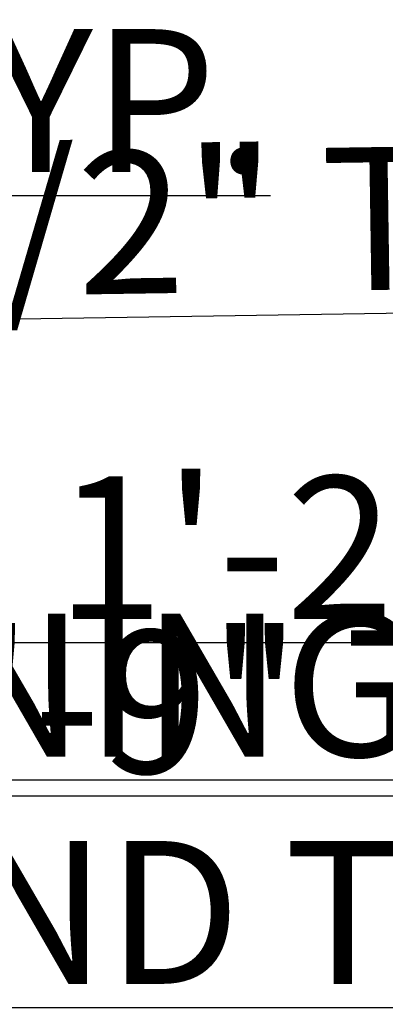
# Model space of a CAD drawing. Units: inches. Extents: x 2901 to 21549, y 2042 to 3828.
# Tile 7 of 10: x 3682 to 3774, y 3099 to 3347. Entities that reach past the tile are written whole.
import ezdxf

# ---------------------------------------------------------------- set-up
doc = ezdxf.new("R2010")
doc.units = ezdxf.units.IN
doc.layers.get('Defpoints').update_dxf_attribs({"color": 1})
doc.layers.add('A-ANNO-DIMS', color=2, linetype='Continuous', lineweight=18)
doc.styles.get("Standard").update_dxf_attribs({"font": 'arial.ttf'})
doc.dimstyles.new('ISO-25', dxfattribs={"dimtxt": 36, "dimasz": 5, "dimexe": 1.25, "dimexo": 0.625, "dimtad": 1, "dimdec": 0, "dimlunit": 3, "dimtxsty": 'Standard', "dimcen": 2.5, "dimadec": 0, "dimazin": 0, "dimtfac": 1, "dimtdec": 0, "dimtmove": 0, "dimatfit": 3, "dimfxl": 1, "dimarcsym": 0})

# ---------------------------------------------------------------- blocks, each defined once
blk = doc.blocks.new('*D36')
at = {"layer": 'A-ANNO-DIMS', "color": 0, "lineweight": -2, "transparency": 16777216}
for p, q in [((3639.47, 3192.64), (3639.47, 3654.44)), ((3634.69, 3192.64), (3640.72, 3192.64)), ((3639.47, 3161.64), (3639.47, 3187.64)), ((3634.69, 3156.64), (3640.72, 3156.64))]:
    blk.add_line(p, q, dxfattribs=at)
at = {"layer": 'A-ANNO-DIMS', "color": 0, "transparency": 16777216}
for points in [[(3638.64, 3187.64), (3640.3, 3187.64), (3639.47, 3192.64)], [(3638.64, 3161.64), (3640.3, 3161.64), (3639.47, 3156.64)]]:
    blk.add_solid(points, dxfattribs=at)
at = {"layer": 'Defpoints', "color": 0, "transparency": 16777216}
for p in [(3634.07, 3192.64), (3639.47, 3192.64), (3634.07, 3156.64)]:
    blk.add_point(p, dxfattribs=at)
at = {"layer": 'A-ANNO-DIMS', "color": 0, "transparency": 16777216, "insert": (3620.21, 3426.04), "char_height": 36, "attachment_point": 5, "rotation": 90}
blk.add_mtext('WINDOW 3\'-0" TYP.', dxfattribs=at)
blk = doc.blocks.new('*D37')
at = {"layer": 'A-ANNO-DIMS', "color": 0, "lineweight": -2, "transparency": 16777216}
for p, q in [((3625.07, 3156.01), (3625.07, 3149.99)), ((3634.07, 3156.01), (3634.07, 3149.99)), ((3620.07, 3151.24), (3615.07, 3151.24)), ((3625.07, 3151.24), (3634.07, 3151.24)), ((3639.07, 3151.24), (3864.76, 3151.24))]:
    blk.add_line(p, q, dxfattribs=at)
at = {"layer": 'A-ANNO-DIMS', "color": 0, "transparency": 16777216}
for points in [[(3620.07, 3152.07), (3620.07, 3150.41), (3625.07, 3151.24)], [(3639.07, 3152.07), (3639.07, 3150.41), (3634.07, 3151.24)]]:
    blk.add_solid(points, dxfattribs=at)
at = {"layer": 'Defpoints', "color": 0, "transparency": 16777216}
for p in [(3625.07, 3156.64), (3634.07, 3156.64), (3634.07, 3151.24)]:
    blk.add_point(p, dxfattribs=at)
at = {"layer": 'A-ANNO-DIMS', "color": 0, "transparency": 16777216, "insert": (3754.41, 3170.24), "char_height": 36, "attachment_point": 5}
blk.add_mtext('0\'-9" TYP.', dxfattribs=at)
blk = doc.blocks.new('*D38')
at = {"layer": 'A-ANNO-DIMS', "color": 0, "lineweight": -2, "transparency": 16777216}
for p, q in [((3343.07, 3191.34), (3343.07, 3188.58)), ((3357.29, 3191.34), (3357.29, 3188.58)), ((3348.07, 3189.83), (3352.29, 3189.83)), ((3357.29, 3189.83), (3922.11, 3189.83))]:
    blk.add_line(p, q, dxfattribs=at)
at = {"layer": 'A-ANNO-DIMS', "color": 0, "transparency": 16777216}
for points in [[(3348.07, 3190.67), (3348.07, 3189), (3343.07, 3189.83)], [(3352.29, 3190.67), (3352.29, 3189), (3357.29, 3189.83)]]:
    blk.add_solid(points, dxfattribs=at)
at = {"layer": 'Defpoints', "color": 0, "transparency": 16777216}
for p in [(3343.07, 3191.97), (3357.29, 3191.97), (3357.29, 3189.83)]:
    blk.add_point(p, dxfattribs=at)
at = {"layer": 'A-ANNO-DIMS', "color": 0, "transparency": 16777216, "insert": (3642.2, 3209.07), "char_height": 36, "attachment_point": 5}
blk.add_mtext('NIGHTSTAND 1\'-2" TYP.', dxfattribs=at)
blk = doc.blocks.new('*D43')
at = {"layer": 'A-ANNO-DIMS', "color": 0, "lineweight": -2, "transparency": 16777216}
for p, q in [((3550.8, 3269.4), (3856.95, 3274.04)), ((3536.1, 3267.11), (3536.05, 3270.42)), ((3541.07, 3269.25), (3545.8, 3269.32)), ((3550.83, 3267.33), (3550.78, 3270.65))]:
    blk.add_line(p, q, dxfattribs=at)
at = {"layer": 'A-ANNO-DIMS', "color": 0, "transparency": 16777216}
for points in [[(3541.06, 3270.08), (3541.09, 3268.42), (3536.07, 3269.17)], [(3545.78, 3270.16), (3545.81, 3268.49), (3550.8, 3269.4)]]:
    blk.add_solid(points, dxfattribs=at)
at = {"layer": 'Defpoints', "color": 0, "transparency": 16777216}
for p in [(3550.8, 3269.4), (3536.11, 3266.48), (3550.84, 3266.71)]:
    blk.add_point(p, dxfattribs=at)
at = {"layer": 'A-ANNO-DIMS', "color": 0, "transparency": 16777216, "insert": (3706.08, 3290.99), "char_height": 36, "attachment_point": 5, "rotation": 0.8679}
blk.add_mtext('1\'-2 1/2" TYP.', dxfattribs=at)
blk = doc.blocks.new('*D45')
at = {"layer": 'A-ANNO-DIMS', "color": 0, "lineweight": -2, "transparency": 16777216}
for p, q in [((3419.19, 3302.47), (3414.19, 3302.47)), ((3424.19, 3301.6), (3424.19, 3303.72)), ((3424.19, 3302.47), (3430.69, 3302.47)), ((3430.69, 3301.6), (3430.69, 3303.72)), ((3435.69, 3302.47), (3745.26, 3302.47))]:
    blk.add_line(p, q, dxfattribs=at)
at = {"layer": 'A-ANNO-DIMS', "color": 0, "transparency": 16777216}
for points in [[(3419.19, 3303.31), (3419.19, 3301.64), (3424.19, 3302.47)], [(3435.69, 3303.31), (3435.69, 3301.64), (3430.69, 3302.47)]]:
    blk.add_solid(points, dxfattribs=at)
at = {"layer": 'Defpoints', "color": 0, "transparency": 16777216}
for p in [(3430.69, 3302.47), (3424.19, 3300.97), (3430.69, 3300.97)]:
    blk.add_point(p, dxfattribs=at)
at = {"layer": 'A-ANNO-DIMS', "color": 0, "transparency": 16777216, "insert": (3592.98, 3321.71), "char_height": 36, "attachment_point": 5}
blk.add_mtext('0\'-6 1/2" TYP.', dxfattribs=at)
blk = doc.blocks.new('*D46')
at = {"layer": 'A-ANNO-DIMS', "color": 0, "lineweight": -2, "transparency": 16777216}
for p, q in [((3545.07, 3370.05), (3545.07, 3357.42)), ((3625.07, 3370.05), (3625.07, 3357.42)), ((3550.07, 3358.67), (3620.07, 3358.67)), ((3625.07, 3358.67), (4160.88, 3358.67))]:
    blk.add_line(p, q, dxfattribs=at)
at = {"layer": 'A-ANNO-DIMS', "color": 0, "transparency": 16777216}
for points in [[(3550.07, 3359.51), (3550.07, 3357.84), (3545.07, 3358.67)], [(3620.07, 3359.51), (3620.07, 3357.84), (3625.07, 3358.67)]]:
    blk.add_solid(points, dxfattribs=at)
at = {"layer": 'Defpoints', "color": 0, "transparency": 16777216}
for p in [(3545.07, 3370.67), (3625.07, 3370.67), (3625.07, 3358.67)]:
    blk.add_point(p, dxfattribs=at)
at = {"layer": 'A-ANNO-DIMS', "color": 0, "transparency": 16777216, "insert": (3895.48, 3379.02), "char_height": 36, "attachment_point": 5}
blk.add_mtext('QUEEN BED 6\'-8" TYP.', dxfattribs=at)
blk = doc.blocks.new('*D48')
at = {"layer": 'A-ANNO-DIMS', "color": 0, "lineweight": -2, "transparency": 16777216}
for p, q in [((3552.33, 3036.58), (3552.33, 3043.43)), ((3557.33, 3042.18), (3588.77, 3042.18)), ((3593.77, 3036.58), (3593.77, 3043.43)), ((3593.77, 3042.18), (4181.25, 3042.18))]:
    blk.add_line(p, q, dxfattribs=at)
at = {"layer": 'A-ANNO-DIMS', "color": 0, "transparency": 16777216}
for points in [[(3557.33, 3043.01), (3557.33, 3041.34), (3552.33, 3042.18)], [(3588.77, 3043.01), (3588.77, 3041.34), (3593.77, 3042.18)]]:
    blk.add_solid(points, dxfattribs=at)
at = {"layer": 'Defpoints', "color": 0, "transparency": 16777216}
for p in [(3593.77, 3042.18), (3552.33, 3035.96), (3593.77, 3035.96)]:
    blk.add_point(p, dxfattribs=at)
at = {"layer": 'A-ANNO-DIMS', "color": 0, "transparency": 16777216, "insert": (3890.01, 3061.44), "char_height": 36, "attachment_point": 5}
blk.add_mtext('LOVESEAT 3\'-5 1/2" TYP.', dxfattribs=at)
blk = doc.blocks.new('*D50')
at = {"layer": 'A-ANNO-DIMS', "color": 0, "lineweight": -2, "transparency": 16777216}
for p, q in [((3599.61, 3100.68), (3599.61, 3096.69)), ((3622.08, 3100.68), (3622.08, 3096.69)), ((3604.61, 3097.94), (3617.08, 3097.94)), ((3622.08, 3097.94), (4251.18, 3097.94))]:
    blk.add_line(p, q, dxfattribs=at)
at = {"layer": 'A-ANNO-DIMS', "color": 0, "transparency": 16777216}
for points in [[(3604.61, 3098.77), (3604.61, 3097.1), (3599.61, 3097.94)], [(3617.08, 3098.77), (3617.08, 3097.1), (3622.08, 3097.94)]]:
    blk.add_solid(points, dxfattribs=at)
at = {"layer": 'Defpoints', "color": 0, "transparency": 16777216}
for p in [(3599.61, 3101.31), (3622.08, 3101.31), (3622.08, 3097.94)]:
    blk.add_point(p, dxfattribs=at)
at = {"layer": 'A-ANNO-DIMS', "color": 0, "transparency": 16777216, "insert": (3939.13, 3117.18), "char_height": 36, "attachment_point": 5}
blk.add_mtext('END TABLE 1\'-10 1/2" TYP.', dxfattribs=at)
blk = doc.blocks.new('*D54')
at = {"layer": 'A-ANNO-DIMS', "color": 0, "lineweight": -2, "transparency": 16777216}
for p, q in [((3536.12, 3164.87), (3536.12, 3153.97)), ((3604.61, 3164.87), (3604.61, 3153.97)), ((3541.12, 3155.22), (3599.61, 3155.22)), ((3604.61, 3155.22), (4090.43, 3155.22))]:
    blk.add_line(p, q, dxfattribs=at)
at = {"layer": 'A-ANNO-DIMS', "color": 0, "transparency": 16777216}
for points in [[(3541.12, 3156.05), (3541.12, 3154.38), (3536.12, 3155.22)], [(3599.61, 3156.05), (3599.61, 3154.38), (3604.61, 3155.22)]]:
    blk.add_solid(points, dxfattribs=at)
at = {"layer": 'Defpoints', "color": 0, "transparency": 16777216}
for p in [(3536.12, 3165.49), (3604.61, 3165.49), (3604.61, 3155.22)]:
    blk.add_point(p, dxfattribs=at)
at = {"layer": 'A-ANNO-DIMS', "color": 0, "transparency": 16777216, "insert": (3850.02, 3174.46), "char_height": 36, "attachment_point": 5}
blk.add_mtext('DINING SET 5\'-8 1/2"', dxfattribs=at)
blk = doc.blocks.new('*D57')
at = {"layer": 'A-ANNO-DIMS', "color": 0, "lineweight": -2, "transparency": 16777216}
for p, q in [((3601.59, 3038.97), (3601.59, 3029.64)), ((3626.91, 3038.97), (3626.91, 3029.64)), ((3606.59, 3030.89), (3621.91, 3030.89)), ((3626.91, 3030.89), (3813.36, 3030.89))]:
    blk.add_line(p, q, dxfattribs=at)
at = {"layer": 'A-ANNO-DIMS', "color": 0, "transparency": 16777216}
for points in [[(3606.59, 3031.73), (3606.59, 3030.06), (3601.59, 3030.89)], [(3621.91, 3031.73), (3621.91, 3030.06), (3626.91, 3030.89)]]:
    blk.add_solid(points, dxfattribs=at)
at = {"layer": 'Defpoints', "color": 0, "transparency": 16777216}
for p in [(3601.59, 3039.6), (3626.91, 3039.6), (3626.91, 3030.89)]:
    blk.add_point(p, dxfattribs=at)
at = {"layer": 'A-ANNO-DIMS', "color": 0, "transparency": 16777216, "insert": (3722.63, 3050.13), "char_height": 36, "attachment_point": 5}
blk.add_mtext('2\'-1 1/2"', dxfattribs=at)
blk = doc.blocks.new('*D73')
at = {"layer": 'A-ANNO-DIMS', "color": 0, "lineweight": -2, "transparency": 16777216}
for p, q in [((3668.02, 3058.19), (3668.02, 3244)), ((3625.69, 3058.19), (3669.27, 3058.19)), ((3668.02, 3017.48), (3668.02, 3053.19)), ((3625.69, 3012.48), (3669.27, 3012.48))]:
    blk.add_line(p, q, dxfattribs=at)
at = {"layer": 'A-ANNO-DIMS', "color": 0, "transparency": 16777216}
for points in [[(3667.19, 3053.19), (3668.85, 3053.19), (3668.02, 3058.19)], [(3667.19, 3017.48), (3668.85, 3017.48), (3668.02, 3012.48)]]:
    blk.add_solid(points, dxfattribs=at)
at = {"layer": 'Defpoints', "color": 0, "transparency": 16777216}
for p in [(3625.07, 3058.19), (3668.02, 3058.19), (3625.07, 3012.48)]:
    blk.add_point(p, dxfattribs=at)
at = {"layer": 'A-ANNO-DIMS', "color": 0, "transparency": 16777216, "insert": (3648.77, 3153.6), "char_height": 36, "attachment_point": 5, "rotation": 90}
blk.add_mtext('3\'-9 1/2"', dxfattribs=at)

msp = doc.modelspace()

# ---------------------------------------------------------------- dimensions: what is measured, and where the dimension line sits
at = {"layer": 'A-ANNO-DIMS'}
for base, p1, p2, angle, text, picture, middle in [((3639.47, 3192.64), (3634.07, 3156.64), (3634.07, 3192.64), 90, 'WINDOW <> TYP.', '*D36', (3620.21, 3426.04)), ((3550.8, 3269.4), (3536.11, 3266.48), (3550.84, 3266.71), 0.8679, '<> TYP.', '*D43', (3706.08, 3290.99))]:
    dim = msp.add_linear_dim(base=base, p1=p1, p2=p2, angle=angle, text=text, dimstyle='ISO-25', override={"dimdec": 1, "dimlfac": 1, "dimrnd": 0, "dimzin": 1, "dimdsep": 46, "dimlunit": 4, "dimfrac": 2}, dxfattribs=at)
    dim.commit()
    dim.dimension.update_dxf_attribs({"geometry": picture, "text_midpoint": middle})
for base, p1, p2, text, picture, middle in [((3625.07, 3358.67), (3545.07, 3370.67), (3625.07, 3370.67), 'QUEEN BED <> TYP.', '*D46', (3895.48, 3379.02)), ((3430.69, 3302.47), (3424.19, 3300.97), (3430.69, 3300.97), '<> TYP.', '*D45', (3592.98, 3321.71)), ((3357.29, 3189.83), (3343.07, 3191.97), (3357.29, 3191.97), 'NIGHTSTAND <> TYP.', '*D38', (3642.2, 3209.07)), ((3604.61, 3155.22), (3536.12, 3165.49), (3604.61, 3165.49), 'DINING SET <>', '*D54', (3850.02, 3174.46)), ((3622.08, 3097.94), (3599.61, 3101.31), (3622.08, 3101.31), 'END TABLE <> TYP.', '*D50', (3939.13, 3117.18)), ((3634.07, 3151.24), (3625.07, 3156.64), (3634.07, 3156.64), '<> TYP.', '*D37', (3754.41, 3170.24)), ((3593.77, 3042.18), (3552.33, 3035.96), (3593.77, 3035.96), 'LOVESEAT <> TYP.', '*D48', (3890.01, 3061.44))]:
    dim = msp.add_linear_dim(base=base, p1=p1, p2=p2, text=text, dimstyle='ISO-25', override={"dimdec": 1, "dimlfac": 1, "dimrnd": 0, "dimzin": 1, "dimdsep": 46, "dimlunit": 4, "dimfrac": 2}, dxfattribs=at)
    dim.commit()
    dim.dimension.update_dxf_attribs({"geometry": picture, "text_midpoint": middle})
dim = msp.add_linear_dim(base=(3668.02, 3058.19), p1=(3625.07, 3012.48), p2=(3625.07, 3058.19), angle=90, dimstyle='ISO-25', override={"dimdec": 1, "dimlfac": 1, "dimrnd": 0, "dimzin": 1, "dimdsep": 46, "dimlunit": 4, "dimfrac": 2}, dxfattribs=at)
dim.commit()
dim.dimension.update_dxf_attribs({"geometry": '*D73', "text_midpoint": (3648.77, 3153.6)})
dim = msp.add_linear_dim(base=(3626.91, 3030.89), p1=(3601.59, 3039.6), p2=(3626.91, 3039.6), dimstyle='ISO-25', override={"dimdec": 1, "dimlfac": 1, "dimrnd": 0, "dimzin": 1, "dimdsep": 46, "dimlunit": 4, "dimfrac": 2}, dxfattribs=at)
dim.commit()
dim.dimension.update_dxf_attribs({"geometry": '*D57', "text_midpoint": (3722.63, 3050.13)})

doc.saveas('drawing.dxf')
